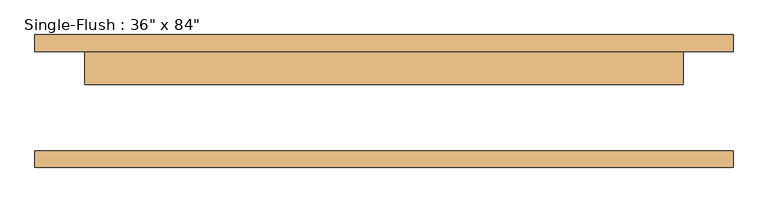
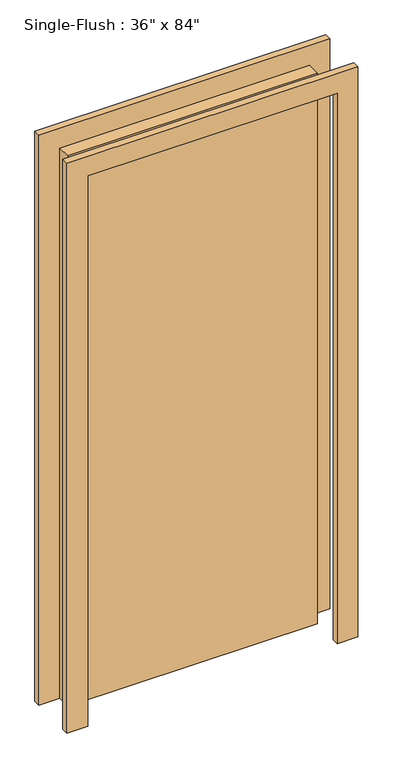
"""IFC4 building model written with IfcOpenShell, lengths in millimetres: door geometry."""

from ifc_helpers import new_model, si_unit, frame, origin, origin_with_axes, place, context, project, spatial, polyline, outline, extrude, source, transform, mapped, element, save


def door_16372e1c(model_context):
    return source(origin(), model_context, "Body", "SweptSolid", [
        extrude(outline(polyline([(2209.8, -533.4), (0.0, -533.4), (0.0, -457.2), (2133.6, -457.2), (2133.6, 457.2), (0.0, 457.2), (0.0, 533.4), (2209.8, 533.4), (2209.8, -533.4)])), frame((0.0, 76.2, 0.0), z_axis=(0.0, 1.0, 0.0), x_axis=(0.0, 0.0, 1.0)), (0.0, 0.0, 1.0), 25.4),
        extrude(outline(polyline([(2209.8, 533.4), (2209.8, -533.4), (0.0, -533.4), (0.0, -457.2), (2133.6, -457.2), (2133.6, 457.2), (0.0, 457.2), (0.0, 533.4), (2209.8, 533.4)])), frame((0.0, -101.6, 0.0), z_axis=(0.0, 1.0, 0.0), x_axis=(0.0, 0.0, 1.0)), (0.0, 0.0, 1.0), 25.4),
        extrude(outline(polyline([(457.2, 25.4), (-457.2, 25.4), (-457.2, 76.2), (457.2, 76.2), (457.2, 25.4)])), origin_with_axes(), (0.0, 0.0, 1.0), 2133.6),
    ])


if __name__ == "__main__":
    model = new_model("IFC4")
    model_context = context("Model", 3, world=origin())
    ifc_project = project(units=[si_unit("LENGTHUNIT", "METRE", prefix="MILLI")], contexts=[model_context])
    site = spatial("IfcSite", under=ifc_project)
    building = spatial("IfcBuilding", under=site)
    placement = place(None, origin())
    door_shape = door_16372e1c(model_context)
    element("IfcDoor", 1, ObjectType="Single-Flush : 36\" x 84\"", at=placement, inside=building, context=model_context, shape_type="MappedRepresentation", body=[
        mapped(door_shape, transform((0.0, 0.0, 0.0), x_axis=(1.0, 0.0, 0.0), y_axis=(0.0, 1.0, 0.0), z_axis=(0.0, 0.0, 1.0))),
    ])
    save(model, "model.ifc")

# Revit data of these elements
# Type "Single-Flush : 36\" x 84\""
#   Type Mark = "1"
#   Construction Type Id = "MDOOR"
#   Assembly Code = "C1020"
#   Analytic Construction = "Metal"
#   Thickness = 0' - 2"
#   Heat Transfer Coefficient (U) = 0.651978 BTU/(h·ft²·°F)
#   Height = 7' - 0"
#   Trim Projection Ext = 0' - 1"
#   Trim Projection Int = 0' - 1"
#   Trim Width = 0' - 3"
#   Width = 3' - 0"
#   Define Thermal Properties by = 1
#   Door Material = Door - Panel
#   Frame Material = Door - Frame
#   Visual Light Transmittance = 0
#   Solar Heat Gain Coefficient = 0
#   Function = (empty or 0)
#   Wall Closure = (empty or 0)
# Element 1 (IfcDoor, "Single-Flush : 36\" x 84\"")
#   Materials on its faces: "Door - Frame", "Door - Panel"
# Materials
#   "Door - Panel": class "Wood", colour RGB 210 159 95, transparency 0
#   "Door - Frame": colour RGB 118 70 51, transparency 0
